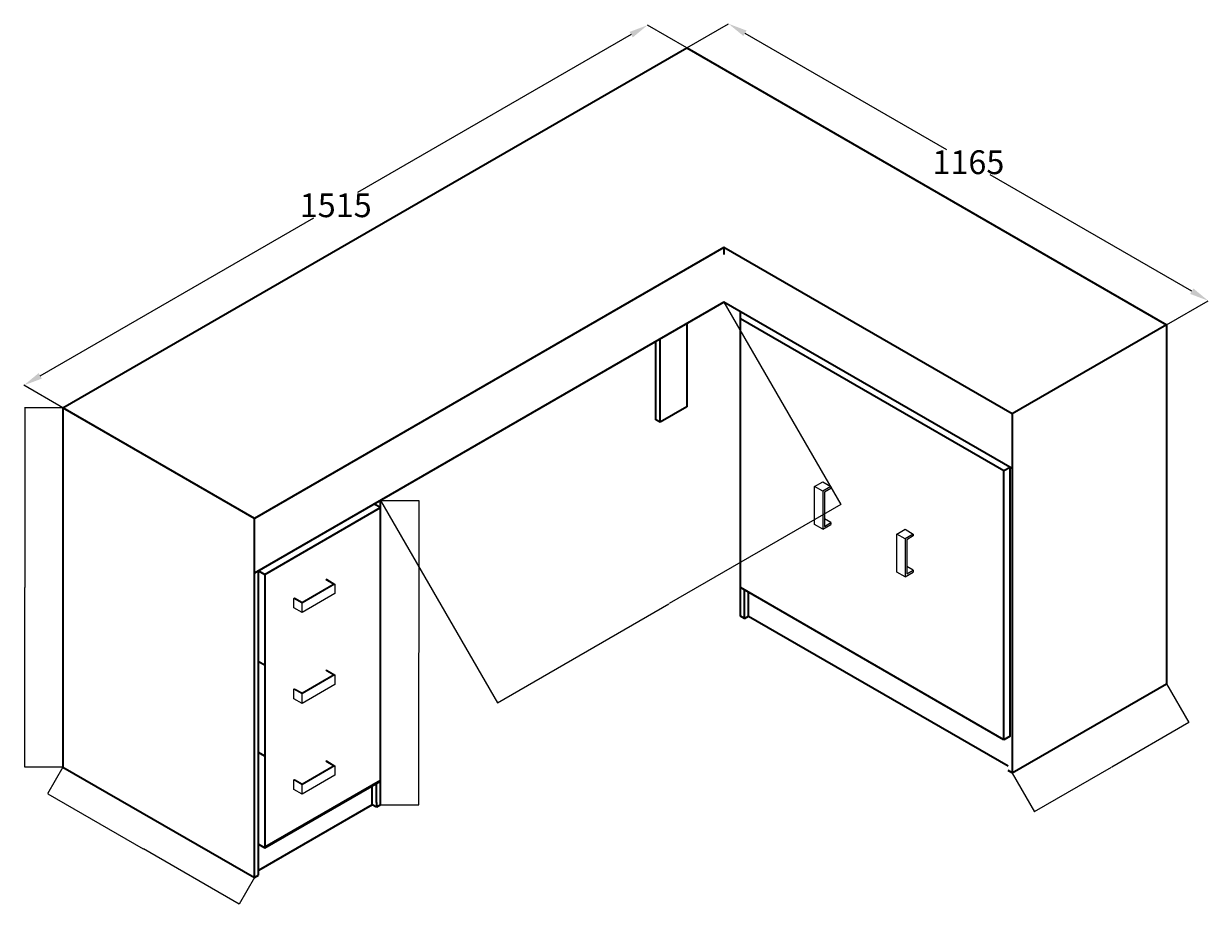
# Model space of a CAD drawing. Units: inches. Extents: x -58 to 51102, y -18784 to 9156.
# Tile 1 of 1: x -58 to 2433, y -1021 to 831. Entities that reach past the tile are written whole.
import ezdxf

# ---------------------------------------------------------------- set-up
doc = ezdxf.new("R2010")
doc.units = ezdxf.units.IN
doc.header["$MEASUREMENT"] = 0
for name, color, linetype, lineweight in [('A-ANNO-DIMS', 2, 'Continuous', 18), ('A-FURN', 7, 'Continuous', 35), ('A-FURN-HRDW', 8, 'Continuous', 18)]:
    doc.layers.add(name, color=color, linetype=linetype, lineweight=lineweight)
doc.styles.get("Standard").update_dxf_attribs({"font": 'arial.ttf'})
doc.dimstyles.get("Standard").update_dxf_attribs({"dimtxt": 0.18, "dimasz": 0.18, "dimexe": 0.18, "dimexo": 0.0625, "dimgap": 0.09, "dimtad": 0, "dimtih": 1, "dimtoh": 1, "dimdec": 0, "dimzin": 0, "dimdsep": 46, "dimtxsty": 'Standard', "dimcen": 0.09, "dimadec": 0, "dimazin": 0, "dimtfac": 1, "dimtdec": 0, "dimtofl": 0, "dimtmove": 0, "dimatfit": 3, "dimfxl": 1, "dimtolj": 1, "dimtzin": 0, "dimarcsym": 0})

# ---------------------------------------------------------------- blocks, each defined once
blk = doc.blocks.new('*D1')
at = {"layer": 'A-ANNO-DIMS', "color": 0, "lineweight": -2, "transparency": 16777216}
for p, q in [((1336.3, 780.5), (1253.8, 828.2)), ((1219.3, 808.1), (644, 475.9)), ((-23.4, 90.6), (551.8, 422.7)), ((24.3, 23), (-58.3, 70.7))]:
    blk.add_line(p, q, dxfattribs=at)
at = {"layer": 'A-ANNO-DIMS', "color": 0, "transparency": 16777216}
for points in [[(1216, 813.9), (1222.6, 802.3), (1253.9, 828.1)], [(-26.8, 96.4), (-20.1, 84.8), (-58.1, 70.6)]]:
    blk.add_solid(points, dxfattribs=at)
at = {"layer": 'Defpoints', "color": 0, "transparency": 16777216}
for p in [(1253.9, 828.1), (1336.4, 780.5), (24.4, 23)]:
    blk.add_point(p, dxfattribs=at)
at = {"layer": 'A-ANNO-DIMS', "color": 0, "transparency": 16777216, "insert": (597.9, 449.3), "char_height": 50, "attachment_point": 5}
blk.add_mtext('\\A1;1515', dxfattribs=at)
blk = doc.blocks.new('*D2')
at = {"layer": 'A-ANNO-DIMS', "color": 0, "lineweight": -2, "transparency": 16777216}
for p, q in [((1336.5, 780.5), (1424.1, 831.1)), ((1458.6, 811), (1882.3, 566.4)), ((2398.2, 268.5), (1974.5, 513.2)), ((2345.4, 198), (2433, 248.6))]:
    blk.add_line(p, q, dxfattribs=at)
at = {"layer": 'A-ANNO-DIMS', "color": 0, "transparency": 16777216}
for points in [[(1461.9, 816.8), (1455.3, 805.3), (1423.9, 831)], [(2401.6, 274.3), (2394.9, 262.8), (2432.9, 248.5)]]:
    blk.add_solid(points, dxfattribs=at)
at = {"layer": 'Defpoints', "color": 0, "transparency": 16777216}
for p in [(1336.4, 780.5), (2432.9, 248.5), (2345.3, 198)]:
    blk.add_point(p, dxfattribs=at)
at = {"layer": 'A-ANNO-DIMS', "color": 0, "transparency": 16777216, "insert": (1928.4, 539.8), "char_height": 50, "attachment_point": 5}
blk.add_mtext('\\A1;1165', dxfattribs=at)
blk = doc.blocks.new('HANDLE-DRAWER')
for p, q in [((86.6, 60), (17.3, 20)), ((17.3, 22), (83.1, 60)), ((69.3, 70), (67.5, 69)), ((83.1, 60), (67.5, 69)), ((69.3, 70), (86.6, 60)), ((86.6, 60), (86.6, 40)), ((0, 30), (1.7, 31)), ((17.3, 20), (0, 30)), ((0, 10), (0, 30)), ((1.7, 31), (17.3, 22)), ((86.6, 40), (17.3, 0)), ((17.3, 0), (0, 10)), ((17.3, 0), (17.3, 20))]:
    blk.add_line(p, q)
blk = doc.blocks.new('HANDLE-DOOR')
for p, q in [((0, 90), (17.3, 100)), ((17.3, 100), (34.6, 90)), ((17.3, 80), (0, 90)), ((0, 10), (0, 90)), ((34.6, 90), (17.3, 80)), ((17.3, 80), (17.3, 0)), ((34.6, 86), (20.8, 78)), ((20.8, 78), (20.8, 6)), ((34.6, 90), (34.6, 86)), ((17.3, 0), (0, 10)), ((17.3, 0), (34.6, 10)), ((34.6, 14), (20.8, 22)), ((20.8, 6), (34.6, 14)), ((34.6, 14), (34.6, 10))]:
    blk.add_line(p, q)
blk = doc.blocks.new('*D5')
at = {"layer": 'A-ANNO-DIMS', "color": 0, "lineweight": -2, "transparency": 16777216}
for p, q in [((24.3, 23), (-56.4, 23)), ((-56.2, 22.8), (-56.2, -354.3)), ((-56.2, -731.8), (-56.2, -354.7)), ((24.3, -732), (-56.4, -732))]:
    blk.add_line(p, q, dxfattribs=at)
at = {"layer": 'A-ANNO-DIMS', "color": 0, "transparency": 16777216}
for points in [[(-56.3, 22.8), (-56.2, 22.8), (-56.2, 23)], [(-56.3, -731.8), (-56.2, -731.8), (-56.2, -732)]]:
    blk.add_solid(points, dxfattribs=at)
at = {"layer": 'Defpoints', "color": 0, "transparency": 16777216}
for p in [(24.4, 23), (-56.2, -732), (24.4, -732)]:
    blk.add_point(p, dxfattribs=at)
at = {"layer": 'A-ANNO-DIMS', "color": 0, "transparency": 16777216, "insert": (-56.2, -354.5), "char_height": 0.18, "attachment_point": 5}
blk.add_mtext('\\A1;30', dxfattribs=at)
blk = doc.blocks.new('*D6')
at = {"layer": 'A-ANNO-DIMS', "color": 0, "lineweight": -2, "transparency": 16777216}
for p, q in [((24.3, -732.1), (-8.1, -788.2)), ((-7.8, -788.2), (193.2, -904.2)), ((394.6, -1020.5), (193.6, -904.4)), ((427, -964.6), (394.6, -1020.7))]:
    blk.add_line(p, q, dxfattribs=at)
at = {"layer": 'A-ANNO-DIMS', "color": 0, "transparency": 16777216}
for points in [[(-7.8, -788.1), (-7.8, -788.2), (-8, -788.1)], [(394.6, -1020.4), (394.5, -1020.5), (394.7, -1020.6)]]:
    blk.add_solid(points, dxfattribs=at)
at = {"layer": 'Defpoints', "color": 0, "transparency": 16777216}
for p in [(24.4, -732), (427.1, -964.5), (394.7, -1020.6)]:
    blk.add_point(p, dxfattribs=at)
at = {"layer": 'A-ANNO-DIMS', "color": 0, "transparency": 16777216, "insert": (193.4, -904.3), "char_height": 0.18, "attachment_point": 5}
blk.add_mtext('\\A1;18', dxfattribs=at)
blk = doc.blocks.new('*D7')
at = {"layer": 'A-ANNO-DIMS', "color": 0, "lineweight": -2, "transparency": 16777216}
for p, q in [((1414.4, 245.4), (1660.1, -180.3)), ((692.1, -171.6), (937.9, -597.3)), ((1659.9, -180.2), (1299.1, -388.5)), ((937.9, -597), (1298.7, -388.7))]:
    blk.add_line(p, q, dxfattribs=at)
at = {"layer": 'A-ANNO-DIMS', "color": 0, "transparency": 16777216}
for points in [[(1659.9, -180.2), (1659.9, -180.2), (1660, -180.1)], [(937.9, -597), (938, -597), (937.8, -597.1)]]:
    blk.add_solid(points, dxfattribs=at)
at = {"layer": 'Defpoints', "color": 0, "transparency": 16777216}
for p in [(1414.3, 245.5), (692.1, -171.5), (1660, -180.1)]:
    blk.add_point(p, dxfattribs=at)
at = {"layer": 'A-ANNO-DIMS', "color": 0, "transparency": 16777216, "insert": (1298.9, -388.6), "char_height": 0.18, "attachment_point": 5}
blk.add_mtext('\\A1;33', dxfattribs=at)
blk = doc.blocks.new('*D8')
at = {"layer": 'A-ANNO-DIMS', "color": 0, "lineweight": -2, "transparency": 16777216}
for p, q in [((692.1, -171.5), (772.8, -171.5)), ((772.6, -171.7), (772.6, -491.3)), ((772.6, -811.3), (772.6, -491.7)), ((692.1, -811.5), (772.8, -811.5))]:
    blk.add_line(p, q, dxfattribs=at)
at = {"layer": 'A-ANNO-DIMS', "color": 0, "transparency": 16777216}
for points in [[(772.5, -171.7), (772.6, -171.7), (772.6, -171.5)], [(772.5, -811.3), (772.6, -811.3), (772.6, -811.5)]]:
    blk.add_solid(points, dxfattribs=at)
at = {"layer": 'Defpoints', "color": 0, "transparency": 16777216}
for p in [(692.1, -171.5), (692.1, -811.5), (772.6, -811.5)]:
    blk.add_point(p, dxfattribs=at)
at = {"layer": 'A-ANNO-DIMS', "color": 0, "transparency": 16777216, "insert": (772.6, -491.5), "char_height": 0.18, "attachment_point": 5}
blk.add_mtext('\\A1;25', dxfattribs=at)
blk = doc.blocks.new('*D9')
at = {"layer": 'A-ANNO-DIMS', "color": 0, "lineweight": -2, "transparency": 16777216}
for p, q in [((2345.3, -557.1), (2392.4, -638.5)), ((2392.1, -638.5), (2230.1, -732)), ((2020.6, -744.6), (2067.6, -826)), ((2067.7, -825.8), (2229.7, -732.3))]:
    blk.add_line(p, q, dxfattribs=at)
at = {"layer": 'A-ANNO-DIMS', "color": 0, "transparency": 16777216}
for points in [[(2392.1, -638.4), (2392.1, -638.5), (2392.3, -638.4)], [(2067.7, -825.8), (2067.7, -825.8), (2067.5, -825.9)]]:
    blk.add_solid(points, dxfattribs=at)
at = {"layer": 'Defpoints', "color": 0, "transparency": 16777216}
for p in [(2345.3, -557), (2392.3, -638.4), (2020.6, -744.5)]:
    blk.add_point(p, dxfattribs=at)
at = {"layer": 'A-ANNO-DIMS', "color": 0, "transparency": 16777216, "insert": (2229.9, -732.1), "char_height": 0.18, "attachment_point": 5}
blk.add_mtext('\\A1;15', dxfattribs=at)

msp = doc.modelspace()

# ---------------------------------------------------------------- linework, layer by layer
at = {"layer": 'A-FURN'}
for p, q in [((24.4, 23), (1336.4, 780.5)), ((1336.4, 780.5), (2345.3, 198)), ((1414.3, 360.5), (427.1, -209.5)), ((2020.6, 10.5), (1414.3, 360.5)), ((1414.3, 360.5), (1414.3, 345.5)), ((1414.3, 245.5), (427.1, -324.5)), ((2020.6, -104.5), (1414.3, 245.5)), ((1449, -414.5), (1449, 225.5)), ((1336.4, 200.5), (1336.4, 25.5)), ((2003.2, -109.5), (1449, 210.5)), ((2345.3, 198), (2020.6, 10.5)), ((2345.3, 198), (2345.3, -557)), ((1271.4, -2), (1271.4, 163)), ((1280.1, -7), (1280.1, 168)), ((1336.4, 25.5), (1280.1, -7)), ((24.4, 23), (24.4, -732)), ((427.1, -209.5), (24.4, 23)), ((2020.6, 10.5), (2020.6, -744.5)), ((1280.1, -7), (1271.4, -2)), ((2016.2, -102), (2003.2, -109.5)), ((2003.2, -674.5), (2003.2, -109.5)), ((2016.2, -667), (2016.2, -102)), ((692.1, -811.5), (692.1, -171.5)), ((448.7, -327), (692.1, -186.5)), ((692.1, -186.5), (679.1, -179)), ((427.1, -964.5), (427.1, -209.5)), ((435.7, -949.5), (435.7, -319.5)), ((435.7, -319.5), (448.7, -327)), ((448.7, -327), (448.7, -902)), ((2003.2, -674.5), (1449, -354.5)), ((1457.6, -419.5), (1457.6, -359.5)), ((1466.3, -414.5), (1466.3, -364.5)), ((1457.6, -419.5), (1449, -414.5)), ((1457.6, -419.5), (1466.3, -414.5)), ((1466.3, -414.5), (2011.9, -729.5)), ((448.7, -518), (435.7, -510.5)), ((2020.6, -744.5), (2345.3, -557)), ((2016.2, -667), (2003.2, -674.5)), ((448.7, -709), (435.7, -701.5)), ((24.4, -732), (427.1, -964.5)), ((2020.6, -744.5), (2011.9, -739.5)), ((448.7, -900), (692.1, -759.5)), ((448.7, -902), (692.1, -761.5)), ((674.8, -811.5), (674.8, -771.5)), ((683.4, -806.5), (683.4, -766.5)), ((674.8, -811.5), (435.7, -949.5)), ((683.4, -816.5), (674.8, -811.5)), ((683.4, -806.5), (683.4, -816.5)), ((692.1, -811.5), (683.4, -816.5)), ((435.7, -894.5), (448.7, -902)), ((427.1, -964.5), (435.7, -959.5)), ((435.7, -959.5), (435.7, -949.5))]:
    msp.add_line(p, q, dxfattribs=at)

# ---------------------------------------------------------------- block references
at = {"layer": 'A-FURN-HRDW'}
for name, p in [('HANDLE-DOOR', (1604.9, -232)), ('HANDLE-DOOR', (1778.1, -332)), ('HANDLE-DRAWER', (509.8, -407.3)), ('HANDLE-DRAWER', (509.8, -598.3)), ('HANDLE-DRAWER', (509.8, -789.3))]:
    msp.add_blockref(name, p, dxfattribs=at)

# ---------------------------------------------------------------- dimensions: what is measured, and where the dimension line sits
at = {"layer": 'A-ANNO-DIMS'}
for p1, p2, distance, picture, middle in [((24.4, 23), (1336.4, 780.5), 82.4, '*D1', (597.9, 449.3)), ((1336.4, 780.5), (2345.3, 198), 87.5, '*D2', (1928.4, 539.8))]:
    dim = msp.add_aligned_dim(p1=p1, p2=p2, distance=distance, dimstyle='Standard', override={"dimtxt": 50, "dimasz": 40, "dimgap": 1.09, "dimclrd": 0, "dimclre": 0, "dimclrt": 0}, dxfattribs=at)
    dim.commit()
    dim.dimension.update_dxf_attribs({"geometry": picture, "text_midpoint": middle})
for base, p1, p2, angle, picture, middle in [((1660, -180.1), (692.1, -171.5), (1414.3, 245.5), 30, '*D7', (1298.9, -388.6)), ((-56.2, -732), (24.4, 23), (24.4, -732), 270, '*D5', (-56.2, -354.5)), ((772.6, -811.5), (692.1, -171.5), (692.1, -811.5), 270, '*D8', (772.6, -491.5)), ((2392.3, -638.4), (2020.6, -744.5), (2345.3, -557), 30, '*D9', (2229.9, -732.1)), ((394.7, -1020.6), (24.4, -732), (427.1, -964.5), 330, '*D6', (193.4, -904.3))]:
    dim = msp.add_linear_dim(base=base, p1=p1, p2=p2, angle=angle, dimstyle='Standard', override={"dimlfac": 0.03937, "dimrnd": 0}, dxfattribs=at)
    dim.commit()
    dim.dimension.update_dxf_attribs({"geometry": picture, "text_midpoint": middle})

doc.saveas('drawing.dxf')
